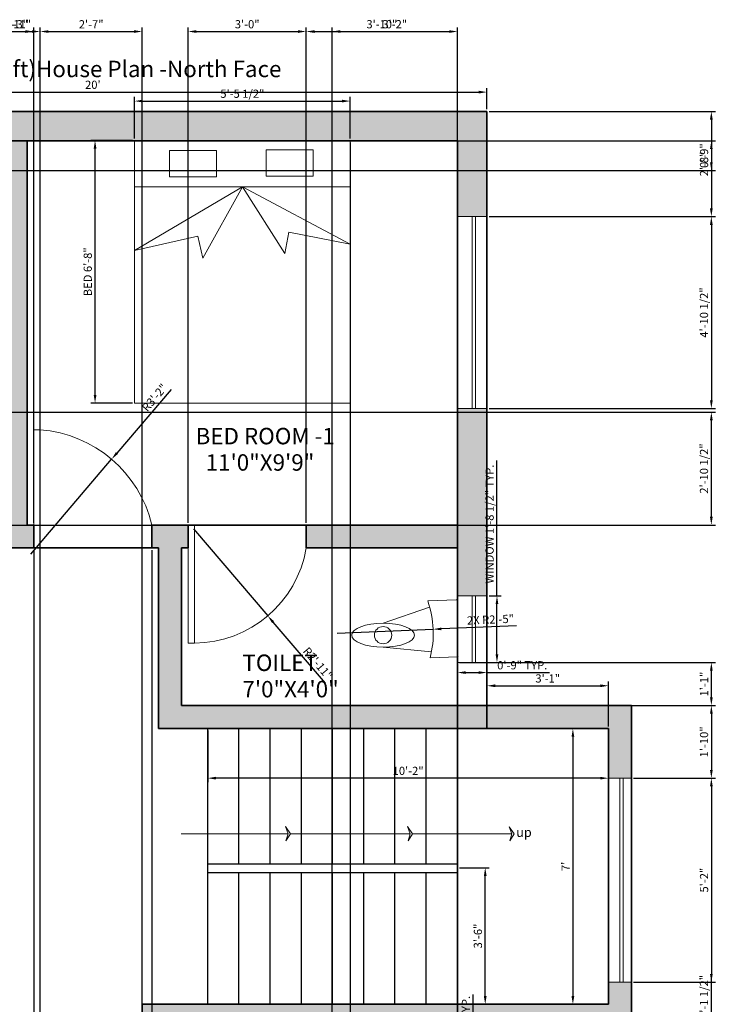
# Model space of a CAD drawing. Units: millimetres. Extents: x 2466 to 2817, y 2000 to 2512.
# Tile 4 of 4: x 2605 to 2817, y 2210 to 2510. Entities that reach past the tile are written whole.
import ezdxf

# ---------------------------------------------------------------- set-up
doc = ezdxf.new("R2010")
doc.units = ezdxf.units.MM
for name, color, linetype, lineweight in [('A-ANNO-DIMS', 2, 'Continuous', 13), ('A-ANNO-SYMB', 1, 'Continuous', 18), ('A-ANNO-TEXT', 7, 'Continuous', 18), ('A-AREA-IDEN', 7, 'Continuous', 18), ('A-DOOR', 3, 'Continuous', 18), ('A-FLOR-FIXT', 9, 'Continuous', 18), ('A-FLOR-STRS', 7, 'Continuous', 25), ('A-FURN', 8, 'Continuous', 18), ('A-GLAZ', 5, 'Continuous', 18), ('A-WALL', 7, 'Continuous', 35), ('A-WALL-PATT', 8, 'Continuous', 13)]:
    doc.layers.add(name, color=color, linetype=linetype, lineweight=lineweight)
doc.styles.get("Standard").update_dxf_attribs({"font": 'arial.ttf'})
doc.dimstyles.new('ISO-25', dxfattribs={"dimtxt": 2.5, "dimasz": 2.5, "dimexe": 1.25, "dimexo": 0.625, "dimtad": 1, "dimdec": 0, "dimlunit": 3, "dimtxsty": 'Standard', "dimcen": 2.5, "dimadec": 0, "dimazin": 0, "dimtfac": 1, "dimtdec": 0, "dimtmove": 0, "dimatfit": 3, "dimfxl": 1, "dimarcsym": 0})

# ---------------------------------------------------------------- blocks, each defined once
blk = doc.blocks.new('MODERN BED')
at = {"color": 0}
for p, q in [((-79.02, 96.24), (0, 96.24)), ((-79.02, 0), (-79.02, 96.24)), ((0, 96.24), (0, 0)), ((0, 79.26), (-79.02, 79.26)), ((-39.51, 79.26), (-79.02, 55.87)), ((-53.99, 53.1), (-39.51, 79.26)), ((-39.51, 79.26), (0, 58.21)), ((-23.98, 54.83), (-39.51, 79.26)), ((-22.46, 62.6), (-23.98, 54.83)), ((0, 58.21), (-22.46, 62.6)), ((-79.02, 55.87), (-55.81, 61.13)), ((-55.81, 61.13), (-53.99, 53.1)), ((0, 0), (-79.02, 0))]:
    blk.add_line(p, q, dxfattribs=at)
for points in [[(-66.19, 92.55), (-48.93, 92.55), (-48.93, 82.91), (-66.19, 82.91)], [(-30.8, 92.85), (-13.54, 92.85), (-13.54, 83.2), (-30.8, 83.2)], [(-30.8, 92.85), (-13.54, 92.85), (-13.54, 83.2), (-30.8, 83.2)]]:
    blk.add_lwpolyline(points, close=True, dxfattribs=at)
blk = doc.blocks.new('*D5')
at = {"layer": 'A-ANNO-DIMS', "color": 0, "lineweight": -2, "transparency": 16777216}
for p, q in [((2738.81, 2251.75), (2747.91, 2251.75)), ((2746.66, 2212.65), (2746.66, 2249.25)), ((2738.81, 2210.15), (2747.91, 2210.15))]:
    blk.add_line(p, q, dxfattribs=at)
at = {"layer": 'A-ANNO-DIMS', "color": 0, "transparency": 16777216}
for points in [[(2746.25, 2249.25), (2747.08, 2249.25), (2746.66, 2251.75)], [(2746.25, 2212.65), (2747.08, 2212.65), (2746.66, 2210.15)]]:
    blk.add_solid(points, dxfattribs=at)
at = {"layer": 'Defpoints', "color": 0, "transparency": 16777216}
for p in [(2738.19, 2251.75), (2746.66, 2251.75), (2738.19, 2210.15)]:
    blk.add_point(p, dxfattribs=at)
at = {"layer": 'A-ANNO-DIMS', "color": 0, "transparency": 16777216, "insert": (2744.76, 2230.95), "char_height": 2.5, "attachment_point": 5, "rotation": 90}
blk.add_mtext('3\'-6"', dxfattribs=at)
blk = doc.blocks.new('*D6')
at = {"layer": 'A-ANNO-DIMS', "color": 0, "lineweight": -2, "transparency": 16777216}
for p, q in [((2783.56, 2294.15), (2772.1, 2294.15)), ((2773.35, 2291.65), (2773.35, 2212.65)), ((2783.56, 2210.15), (2772.1, 2210.15))]:
    blk.add_line(p, q, dxfattribs=at)
at = {"layer": 'A-ANNO-DIMS', "color": 0, "transparency": 16777216}
for points in [[(2772.94, 2291.65), (2773.77, 2291.65), (2773.35, 2294.15)], [(2772.94, 2212.65), (2773.77, 2212.65), (2773.35, 2210.15)]]:
    blk.add_solid(points, dxfattribs=at)
at = {"layer": 'Defpoints', "color": 0, "transparency": 16777216}
for p in [(2784.19, 2294.15), (2773.35, 2210.15), (2784.19, 2210.15)]:
    blk.add_point(p, dxfattribs=at)
at = {"layer": 'A-ANNO-DIMS', "color": 0, "transparency": 16777216, "insert": (2771.48, 2252.15), "char_height": 2.5, "attachment_point": 5, "rotation": 90}
blk.add_mtext("7'", dxfattribs=at)
blk = doc.blocks.new('*D7')
at = {"layer": 'A-ANNO-DIMS', "color": 0, "lineweight": -2, "transparency": 16777216}
for p, q in [((2747.19, 2294.77), (2747.19, 2308.43)), ((2749.69, 2307.18), (2781.69, 2307.18)), ((2784.19, 2294.77), (2784.19, 2308.43))]:
    blk.add_line(p, q, dxfattribs=at)
at = {"layer": 'A-ANNO-DIMS', "color": 0, "transparency": 16777216}
for points in [[(2749.69, 2307.6), (2749.69, 2306.77), (2747.19, 2307.18)], [(2781.69, 2307.6), (2781.69, 2306.77), (2784.19, 2307.18)]]:
    blk.add_solid(points, dxfattribs=at)
at = {"layer": 'Defpoints', "color": 0, "transparency": 16777216}
for p in [(2784.19, 2307.18), (2747.19, 2294.15), (2784.19, 2294.15)]:
    blk.add_point(p, dxfattribs=at)
at = {"layer": 'A-ANNO-DIMS', "color": 0, "transparency": 16777216, "insert": (2765.69, 2309.09), "char_height": 2.5, "attachment_point": 5}
blk.add_mtext('3\'-1"', dxfattribs=at)
blk = doc.blocks.new('*D8')
at = {"layer": 'A-ANNO-DIMS', "color": 0, "lineweight": -2, "transparency": 16777216}
for p, q in [((2662.19, 2293.52), (2662.19, 2277.78)), ((2784.19, 2293.52), (2784.19, 2277.78)), ((2781.69, 2279.03), (2664.69, 2279.03))]:
    blk.add_line(p, q, dxfattribs=at)
at = {"layer": 'A-ANNO-DIMS', "color": 0, "transparency": 16777216}
for points in [[(2664.69, 2279.45), (2664.69, 2278.62), (2662.19, 2279.03)], [(2781.69, 2279.45), (2781.69, 2278.62), (2784.19, 2279.03)]]:
    blk.add_solid(points, dxfattribs=at)
at = {"layer": 'Defpoints', "color": 0, "transparency": 16777216}
for p in [(2662.19, 2294.15), (2784.19, 2294.15), (2662.19, 2279.03)]:
    blk.add_point(p, dxfattribs=at)
at = {"layer": 'A-ANNO-DIMS', "color": 0, "transparency": 16777216, "insert": (2723.19, 2280.93), "char_height": 2.5, "attachment_point": 5}
blk.add_mtext('10\'-2"', dxfattribs=at)
blk = doc.blocks.new('*D9')
at = {"layer": 'A-ANNO-DIMS', "color": 0, "lineweight": -2, "transparency": 16777216}
for p, q in [((2507.19, 2482.77), (2507.19, 2489.26)), ((2509.69, 2488.01), (2744.69, 2488.01)), ((2747.19, 2482.77), (2747.19, 2489.26))]:
    blk.add_line(p, q, dxfattribs=at)
at = {"layer": 'A-ANNO-DIMS', "color": 0, "transparency": 16777216}
for points in [[(2509.69, 2488.43), (2509.69, 2487.6), (2507.19, 2488.01)], [(2744.69, 2488.43), (2744.69, 2487.6), (2747.19, 2488.01)]]:
    blk.add_solid(points, dxfattribs=at)
at = {"layer": 'Defpoints', "color": 0, "transparency": 16777216}
for p in [(2747.19, 2488.01), (2507.19, 2482.15), (2747.19, 2482.15)]:
    blk.add_point(p, dxfattribs=at)
at = {"layer": 'A-ANNO-DIMS', "color": 0, "transparency": 16777216, "insert": (2627.19, 2489.92), "char_height": 2.5, "attachment_point": 5}
blk.add_mtext("20'", dxfattribs=at)
blk = doc.blocks.new('*D10')
at = {"layer": 'A-ANNO-DIMS', "color": 0, "lineweight": -2, "transparency": 16777216}
for p, q in [((2746.56, 2482.15), (2467.98, 2482.15)), ((2469.23, 2479.65), (2469.23, 2028.65)), ((2746.56, 2026.15), (2467.98, 2026.15))]:
    blk.add_line(p, q, dxfattribs=at)
at = {"layer": 'A-ANNO-DIMS', "color": 0, "transparency": 16777216}
for points in [[(2468.82, 2479.65), (2469.65, 2479.65), (2469.23, 2482.15)], [(2468.82, 2028.65), (2469.65, 2028.65), (2469.23, 2026.15)]]:
    blk.add_solid(points, dxfattribs=at)
at = {"layer": 'Defpoints', "color": 0, "transparency": 16777216}
for p in [(2747.19, 2482.15), (2469.23, 2026.15), (2747.19, 2026.15)]:
    blk.add_point(p, dxfattribs=at)
at = {"layer": 'A-ANNO-DIMS', "color": 0, "transparency": 16777216, "insert": (2467.33, 2254.15), "char_height": 2.5, "attachment_point": 5, "rotation": 90}
blk.add_mtext("38'", dxfattribs=at)
blk = doc.blocks.new('WC-PLAN')
for p, q in [((23.74, 15.5), (9.57, 10.55)), ((23.15, 17.36), (31.83, 17.72)), ((24.29, 1.87), (9.58, 3.3)), ((32.19, 0.34), (23.86, 0))]:
    blk.add_line(p, q)
blk.add_circle((9.58, 6.93), 2.64)
blk.add_arc((-4.38, 7.53), 29.23, 345.0736, 19.6488)
blk.add_ellipse((9.58, 6.93), major_axis=(9.58, 0.01), ratio=0.378572)
blk = doc.blocks.new('WIN-BATH')
for p, q in [((4.5, 20.33), (4.5, 0)), ((5.5, 20.33), (5.5, 0))]:
    blk.add_line(p, q)
blk.add_lwpolyline([(9, 20.33), (0, 20.33), (0, 0), (9, 0)], close=True)
blk = doc.blocks.new('STAIR-DIRECTION-HEAD')
blk.add_lwpolyline([(0, 4.35), (0.84, 2.19), (0.16, 0), (1.53, 2.19)], close=True)
blk = doc.blocks.new('*D18')
at = {"layer": 'A-ANNO-DIMS', "color": 0, "lineweight": -2, "transparency": 16777216}
for p, q in [((2750.24, 2334.57), (2750.24, 2375.78)), ((2747.81, 2334.57), (2751.49, 2334.57)), ((2750.24, 2316.74), (2750.24, 2332.07)), ((2747.81, 2314.24), (2751.49, 2314.24))]:
    blk.add_line(p, q, dxfattribs=at)
at = {"layer": 'A-ANNO-DIMS', "color": 0, "transparency": 16777216}
for points in [[(2749.82, 2332.07), (2750.65, 2332.07), (2750.24, 2334.57)], [(2749.82, 2316.74), (2750.65, 2316.74), (2750.24, 2314.24)]]:
    blk.add_solid(points, dxfattribs=at)
at = {"layer": 'Defpoints', "color": 0, "transparency": 16777216}
for p in [(2747.19, 2334.57), (2750.24, 2334.57), (2747.19, 2314.24)]:
    blk.add_point(p, dxfattribs=at)
at = {"layer": 'A-ANNO-DIMS', "color": 0, "transparency": 16777216, "insert": (2748.32, 2356.43), "char_height": 2.5, "attachment_point": 5, "rotation": 90}
blk.add_mtext('WINDOW 1\'-8 1/2" TYP.', dxfattribs=at)
blk = doc.blocks.new('*D19')
at = {"layer": 'A-ANNO-DIMS', "color": 0, "lineweight": -2, "transparency": 16777216}
for p, q in [((2738.19, 2313.62), (2738.19, 2309.95)), ((2747.19, 2313.62), (2747.19, 2309.95)), ((2740.69, 2311.2), (2744.69, 2311.2)), ((2747.19, 2311.2), (2766.18, 2311.2))]:
    blk.add_line(p, q, dxfattribs=at)
at = {"layer": 'A-ANNO-DIMS', "color": 0, "transparency": 16777216}
for points in [[(2740.69, 2311.61), (2740.69, 2310.78), (2738.19, 2311.2)], [(2744.69, 2311.61), (2744.69, 2310.78), (2747.19, 2311.2)]]:
    blk.add_solid(points, dxfattribs=at)
at = {"layer": 'Defpoints', "color": 0, "transparency": 16777216}
for p in [(2738.19, 2314.24), (2747.19, 2314.24), (2747.19, 2311.2)]:
    blk.add_point(p, dxfattribs=at)
at = {"layer": 'A-ANNO-DIMS', "color": 0, "transparency": 16777216, "insert": (2757.93, 2313.1), "char_height": 2.5, "attachment_point": 5}
blk.add_mtext('0\'-9" TYP.', dxfattribs=at)
blk = doc.blocks.new('*D21')
at = {"layer": 'A-ANNO-DIMS', "color": 0, "lineweight": -2, "transparency": 16777216}
for p, q in [((2743.02, 2188.59), (2743.02, 2213.17)), ((2738.81, 2188.59), (2744.27, 2188.59)), ((2743.02, 2173.37), (2743.02, 2186.09)), ((2738.81, 2170.87), (2744.27, 2170.87))]:
    blk.add_line(p, q, dxfattribs=at)
at = {"layer": 'A-ANNO-DIMS', "color": 0, "transparency": 16777216}
for points in [[(2742.6, 2186.09), (2743.43, 2186.09), (2743.02, 2188.59)], [(2742.6, 2173.37), (2743.43, 2173.37), (2743.02, 2170.87)]]:
    blk.add_solid(points, dxfattribs=at)
at = {"layer": 'Defpoints', "color": 0, "transparency": 16777216}
for p in [(2738.19, 2188.59), (2743.02, 2188.59), (2738.19, 2170.87)]:
    blk.add_point(p, dxfattribs=at)
at = {"layer": 'A-ANNO-DIMS', "color": 0, "transparency": 16777216, "insert": (2741.1, 2202.13), "char_height": 2.5, "attachment_point": 5, "rotation": 90}
blk.add_mtext('1\'-5 1/2" TYP.', dxfattribs=at)
blk = doc.blocks.new('*D24')
at = {"layer": 'A-ANNO-DIMS', "color": 0, "lineweight": -2, "transparency": 16777216}
for p, q in [((2639.25, 2473.28), (2626.62, 2473.28)), ((2627.87, 2395.78), (2627.87, 2470.78)), ((2639.25, 2393.28), (2626.62, 2393.28))]:
    blk.add_line(p, q, dxfattribs=at)
at = {"layer": 'A-ANNO-DIMS', "color": 0, "transparency": 16777216}
for points in [[(2627.45, 2470.78), (2628.29, 2470.78), (2627.87, 2473.28)], [(2627.45, 2395.78), (2628.29, 2395.78), (2627.87, 2393.28)]]:
    blk.add_solid(points, dxfattribs=at)
at = {"layer": 'Defpoints', "color": 0, "transparency": 16777216}
for p in [(2627.87, 2473.28), (2639.87, 2473.28), (2639.87, 2393.28)]:
    blk.add_point(p, dxfattribs=at)
at = {"layer": 'A-ANNO-DIMS', "color": 0, "transparency": 16777216, "insert": (2625.97, 2433.28), "char_height": 2.5, "attachment_point": 5, "rotation": 90}
blk.add_mtext('BED 6\'-8"', dxfattribs=at)
blk = doc.blocks.new('*D25')
at = {"layer": 'A-ANNO-DIMS', "color": 0, "lineweight": -2, "transparency": 16777216}
for p, q in [((2639.87, 2473.91), (2639.87, 2486.53)), ((2705.56, 2473.91), (2705.56, 2486.53)), ((2642.37, 2485.28), (2703.06, 2485.28))]:
    blk.add_line(p, q, dxfattribs=at)
at = {"layer": 'A-ANNO-DIMS', "color": 0, "transparency": 16777216}
for points in [[(2642.37, 2485.7), (2642.37, 2484.87), (2639.87, 2485.28)], [(2703.06, 2485.7), (2703.06, 2484.87), (2705.56, 2485.28)]]:
    blk.add_solid(points, dxfattribs=at)
at = {"layer": 'Defpoints', "color": 0, "transparency": 16777216}
for p in [(2705.56, 2485.28), (2639.87, 2473.28), (2705.56, 2473.28)]:
    blk.add_point(p, dxfattribs=at)
at = {"layer": 'A-ANNO-DIMS', "color": 0, "transparency": 16777216, "insert": (2672.72, 2487.2), "char_height": 2.5, "attachment_point": 5}
blk.add_mtext('5\'-5 1/2"', dxfattribs=at)
blk = doc.blocks.new('*D36')
at = {"layer": 'A-ANNO-DIMS', "color": 0, "lineweight": -2, "transparency": 16777216}
for p, q in [((2747.81, 2482.15), (2816.76, 2482.15)), ((2815.51, 2479.65), (2815.51, 2452.58)), ((2747.81, 2450.08), (2816.76, 2450.08))]:
    blk.add_line(p, q, dxfattribs=at)
at = {"layer": 'A-ANNO-DIMS', "color": 0, "transparency": 16777216}
for points in [[(2815.09, 2479.65), (2815.92, 2479.65), (2815.51, 2482.15)], [(2815.09, 2452.58), (2815.92, 2452.58), (2815.51, 2450.08)]]:
    blk.add_solid(points, dxfattribs=at)
at = {"layer": 'Defpoints', "color": 0, "transparency": 16777216}
for p in [(2747.19, 2482.15), (2747.19, 2450.08), (2815.51, 2450.08)]:
    blk.add_point(p, dxfattribs=at)
at = {"layer": 'A-ANNO-DIMS', "color": 0, "transparency": 16777216, "insert": (2813.61, 2466.12), "char_height": 2.5, "attachment_point": 5, "rotation": 90}
blk.add_mtext('2\'-8"', dxfattribs=at)
blk = doc.blocks.new('*D37')
at = {"layer": 'A-ANNO-DIMS', "color": 0, "lineweight": -2, "transparency": 16777216}
for p, q in [((2747.81, 2450.08), (2816.76, 2450.08)), ((2815.51, 2447.58), (2815.51, 2394.15)), ((2747.81, 2391.65), (2816.76, 2391.65))]:
    blk.add_line(p, q, dxfattribs=at)
at = {"layer": 'A-ANNO-DIMS', "color": 0, "transparency": 16777216}
for points in [[(2815.09, 2447.58), (2815.92, 2447.58), (2815.51, 2450.08)], [(2815.09, 2394.15), (2815.92, 2394.15), (2815.51, 2391.65)]]:
    blk.add_solid(points, dxfattribs=at)
at = {"layer": 'Defpoints', "color": 0, "transparency": 16777216}
for p in [(2747.19, 2450.08), (2747.19, 2391.65), (2815.51, 2391.65)]:
    blk.add_point(p, dxfattribs=at)
at = {"layer": 'A-ANNO-DIMS', "color": 0, "transparency": 16777216, "insert": (2813.59, 2420.87), "char_height": 2.5, "attachment_point": 5, "rotation": 90}
blk.add_mtext('4\'-10 1/2"', dxfattribs=at)
blk = doc.blocks.new('*D38')
at = {"layer": 'A-ANNO-DIMS', "color": 0, "lineweight": -2, "transparency": 16777216}
for p, q in [((2791.81, 2301.15), (2816.76, 2301.15)), ((2815.51, 2298.65), (2815.51, 2281.53)), ((2791.81, 2279.03), (2816.76, 2279.03))]:
    blk.add_line(p, q, dxfattribs=at)
at = {"layer": 'A-ANNO-DIMS', "color": 0, "transparency": 16777216}
for points in [[(2815.09, 2298.65), (2815.92, 2298.65), (2815.51, 2301.15)], [(2815.09, 2281.53), (2815.92, 2281.53), (2815.51, 2279.03)]]:
    blk.add_solid(points, dxfattribs=at)
at = {"layer": 'Defpoints', "color": 0, "transparency": 16777216}
for p in [(2791.19, 2301.15), (2791.19, 2279.03), (2815.51, 2279.03)]:
    blk.add_point(p, dxfattribs=at)
at = {"layer": 'A-ANNO-DIMS', "color": 0, "transparency": 16777216, "insert": (2813.61, 2290.09), "char_height": 2.5, "attachment_point": 5, "rotation": 90}
blk.add_mtext('1\'-10"', dxfattribs=at)
blk = doc.blocks.new('*D39')
at = {"layer": 'A-ANNO-DIMS', "color": 0, "lineweight": -2, "transparency": 16777216}
for p, q in [((2791.81, 2279.03), (2816.76, 2279.03)), ((2815.51, 2276.53), (2815.51, 2219.4)), ((2791.81, 2216.9), (2816.76, 2216.9))]:
    blk.add_line(p, q, dxfattribs=at)
at = {"layer": 'A-ANNO-DIMS', "color": 0, "transparency": 16777216}
for points in [[(2815.09, 2276.53), (2815.92, 2276.53), (2815.51, 2279.03)], [(2815.09, 2219.4), (2815.92, 2219.4), (2815.51, 2216.9)]]:
    blk.add_solid(points, dxfattribs=at)
at = {"layer": 'Defpoints', "color": 0, "transparency": 16777216}
for p in [(2791.19, 2279.03), (2791.19, 2216.9), (2815.51, 2216.9)]:
    blk.add_point(p, dxfattribs=at)
at = {"layer": 'A-ANNO-DIMS', "color": 0, "transparency": 16777216, "insert": (2813.61, 2247.97), "char_height": 2.5, "attachment_point": 5, "rotation": 90}
blk.add_mtext('5\'-2"', dxfattribs=at)
blk = doc.blocks.new('*D43')
at = {"layer": 'A-ANNO-DIMS', "color": 0, "lineweight": -2, "transparency": 16777216}
for p, q in [((2700.05, 2035.77), (2700.05, 2507.72)), ((2738.19, 2035.77), (2738.19, 2507.72)), ((2702.55, 2506.47), (2735.69, 2506.47))]:
    blk.add_line(p, q, dxfattribs=at)
at = {"layer": 'A-ANNO-DIMS', "color": 0, "transparency": 16777216}
for points in [[(2702.55, 2506.88), (2702.55, 2506.05), (2700.05, 2506.47)], [(2735.69, 2506.88), (2735.69, 2506.05), (2738.19, 2506.47)]]:
    blk.add_solid(points, dxfattribs=at)
at = {"layer": 'Defpoints', "color": 0, "transparency": 16777216}
for p in [(2738.19, 2506.47), (2700.05, 2035.15), (2738.19, 2035.15)]:
    blk.add_point(p, dxfattribs=at)
at = {"layer": 'A-ANNO-DIMS', "color": 0, "transparency": 16777216, "insert": (2719.12, 2508.37), "char_height": 2.5, "attachment_point": 5}
blk.add_mtext('3\'-2"', dxfattribs=at)
blk = doc.blocks.new('*D49')
at = {"layer": 'A-ANNO-DIMS', "color": 0, "lineweight": -2, "transparency": 16777216}
for p, q in [((2598.19, 2356.77), (2598.19, 2507.72)), ((2609.19, 2356.77), (2609.19, 2507.72)), ((2600.69, 2506.47), (2606.69, 2506.47))]:
    blk.add_line(p, q, dxfattribs=at)
at = {"layer": 'A-ANNO-DIMS', "color": 0, "transparency": 16777216}
for points in [[(2600.69, 2506.88), (2600.69, 2506.05), (2598.19, 2506.47)], [(2606.69, 2506.88), (2606.69, 2506.05), (2609.19, 2506.47)]]:
    blk.add_solid(points, dxfattribs=at)
at = {"layer": 'Defpoints', "color": 0, "transparency": 16777216}
for p in [(2609.19, 2506.47), (2598.19, 2356.15), (2609.19, 2356.15)]:
    blk.add_point(p, dxfattribs=at)
at = {"layer": 'A-ANNO-DIMS', "color": 0, "transparency": 16777216, "insert": (2603.69, 2508.37), "char_height": 2.5, "attachment_point": 5}
blk.add_mtext('0\'-11"', dxfattribs=at)
blk = doc.blocks.new('*D50')
at = {"layer": 'A-ANNO-DIMS', "color": 0, "lineweight": -2, "transparency": 16777216}
for p, q in [((2609.19, 2348.52), (2609.19, 2000.58)), ((2645.19, 2348.52), (2645.19, 2000.58)), ((2611.69, 2001.83), (2642.69, 2001.83))]:
    blk.add_line(p, q, dxfattribs=at)
at = {"layer": 'A-ANNO-DIMS', "color": 0, "transparency": 16777216}
for points in [[(2611.69, 2002.24), (2611.69, 2001.41), (2609.19, 2001.83)], [(2642.69, 2002.24), (2642.69, 2001.41), (2645.19, 2001.83)]]:
    blk.add_solid(points, dxfattribs=at)
at = {"layer": 'Defpoints', "color": 0, "transparency": 16777216}
for p in [(2609.19, 2349.15), (2645.19, 2349.15), (2645.19, 2001.83)]:
    blk.add_point(p, dxfattribs=at)
at = {"layer": 'A-ANNO-DIMS', "color": 0, "transparency": 16777216, "insert": (2627.19, 2003.73), "char_height": 2.5, "attachment_point": 5}
blk.add_mtext('3\'-0"', dxfattribs=at)
blk = doc.blocks.new('*D53')
at = {"layer": 'A-ANNO-DIMS', "color": 0, "lineweight": -2, "transparency": 16777216}
for p, q in [((2596.19, 2155.77), (2596.19, 2507.72)), ((2611.19, 2155.77), (2611.19, 2507.72)), ((2598.69, 2506.47), (2608.69, 2506.47))]:
    blk.add_line(p, q, dxfattribs=at)
at = {"layer": 'A-ANNO-DIMS', "color": 0, "transparency": 16777216}
for points in [[(2598.69, 2506.88), (2598.69, 2506.05), (2596.19, 2506.47)], [(2608.69, 2506.88), (2608.69, 2506.05), (2611.19, 2506.47)]]:
    blk.add_solid(points, dxfattribs=at)
at = {"layer": 'Defpoints', "color": 0, "transparency": 16777216}
for p in [(2611.19, 2506.47), (2596.19, 2155.15), (2611.19, 2155.15)]:
    blk.add_point(p, dxfattribs=at)
at = {"layer": 'A-ANNO-DIMS', "color": 0, "transparency": 16777216, "insert": (2603.69, 2508.37), "char_height": 2.5, "attachment_point": 5}
blk.add_mtext('1\'-3"', dxfattribs=at)
blk = doc.blocks.new('*D54')
at = {"layer": 'A-ANNO-DIMS', "color": 0, "lineweight": -2, "transparency": 16777216}
for p, q in [((2611.19, 2155.77), (2611.19, 2507.72)), ((2642.19, 2155.77), (2642.19, 2507.72)), ((2613.69, 2506.47), (2639.69, 2506.47))]:
    blk.add_line(p, q, dxfattribs=at)
at = {"layer": 'A-ANNO-DIMS', "color": 0, "transparency": 16777216}
for points in [[(2613.69, 2506.88), (2613.69, 2506.05), (2611.19, 2506.47)], [(2639.69, 2506.88), (2639.69, 2506.05), (2642.19, 2506.47)]]:
    blk.add_solid(points, dxfattribs=at)
at = {"layer": 'Defpoints', "color": 0, "transparency": 16777216}
for p in [(2642.19, 2506.47), (2611.19, 2155.15), (2642.19, 2155.15)]:
    blk.add_point(p, dxfattribs=at)
at = {"layer": 'A-ANNO-DIMS', "color": 0, "transparency": 16777216, "insert": (2626.69, 2508.35), "char_height": 2.5, "attachment_point": 5}
blk.add_mtext('2\'-7"', dxfattribs=at)
blk = doc.blocks.new('*D57')
at = {"layer": 'A-ANNO-DIMS', "color": 0, "lineweight": -2, "transparency": 16777216}
for p, q in [((2815.51, 2203.15), (2815.51, 2219.13)), ((2747.81, 2203.15), (2816.76, 2203.15)), ((2815.51, 2192.2), (2815.51, 2200.65)), ((2747.81, 2189.7), (2816.76, 2189.7))]:
    blk.add_line(p, q, dxfattribs=at)
at = {"layer": 'A-ANNO-DIMS', "color": 0, "transparency": 16777216}
for points in [[(2815.09, 2200.65), (2815.92, 2200.65), (2815.51, 2203.15)], [(2815.09, 2192.2), (2815.92, 2192.2), (2815.51, 2189.7)]]:
    blk.add_solid(points, dxfattribs=at)
at = {"layer": 'Defpoints', "color": 0, "transparency": 16777216}
for p in [(2747.19, 2203.15), (2815.51, 2203.15), (2747.19, 2189.7)]:
    blk.add_point(p, dxfattribs=at)
at = {"layer": 'A-ANNO-DIMS', "color": 0, "transparency": 16777216, "insert": (2813.59, 2212.39), "char_height": 2.5, "attachment_point": 5, "rotation": 90}
blk.add_mtext('1\'-1 1/2"', dxfattribs=at)
blk = doc.blocks.new('*D58')
at = {"layer": 'A-ANNO-DIMS', "color": 0, "lineweight": -2, "transparency": 16777216}
for p, q in [((2738.81, 2314.24), (2816.76, 2314.24)), ((2815.51, 2303.65), (2815.51, 2311.74)), ((2738.81, 2301.15), (2816.76, 2301.15))]:
    blk.add_line(p, q, dxfattribs=at)
at = {"layer": 'A-ANNO-DIMS', "color": 0, "transparency": 16777216}
for points in [[(2815.09, 2311.74), (2815.92, 2311.74), (2815.51, 2314.24)], [(2815.09, 2303.65), (2815.92, 2303.65), (2815.51, 2301.15)]]:
    blk.add_solid(points, dxfattribs=at)
at = {"layer": 'Defpoints', "color": 0, "transparency": 16777216}
for p in [(2738.19, 2314.24), (2815.51, 2314.24), (2738.19, 2301.15)]:
    blk.add_point(p, dxfattribs=at)
at = {"layer": 'A-ANNO-DIMS', "color": 0, "transparency": 16777216, "insert": (2813.63, 2307.7), "char_height": 2.5, "attachment_point": 5, "rotation": 90}
blk.add_mtext('1\'-1"', dxfattribs=at)
blk = doc.blocks.new('*D60')
at = {"layer": 'A-ANNO-DIMS', "color": 0, "lineweight": -2, "transparency": 16777216}
for p, q in [((2656.19, 2356.77), (2656.19, 2507.72)), ((2692.19, 2356.77), (2692.19, 2507.72)), ((2658.69, 2506.47), (2689.69, 2506.47))]:
    blk.add_line(p, q, dxfattribs=at)
at = {"layer": 'A-ANNO-DIMS', "color": 0, "transparency": 16777216}
for points in [[(2658.69, 2506.88), (2658.69, 2506.05), (2656.19, 2506.47)], [(2689.69, 2506.88), (2689.69, 2506.05), (2692.19, 2506.47)]]:
    blk.add_solid(points, dxfattribs=at)
at = {"layer": 'Defpoints', "color": 0, "transparency": 16777216}
for p in [(2692.19, 2506.47), (2656.19, 2356.15), (2692.19, 2356.15)]:
    blk.add_point(p, dxfattribs=at)
at = {"layer": 'A-ANNO-DIMS', "color": 0, "transparency": 16777216, "insert": (2674.19, 2508.37), "char_height": 2.5, "attachment_point": 5}
blk.add_mtext('3\'-0"', dxfattribs=at)
blk = doc.blocks.new('*D61')
at = {"layer": 'A-ANNO-DIMS', "color": 0, "lineweight": -2, "transparency": 16777216}
for p, q in [((2692.19, 2356.77), (2692.19, 2507.72)), ((2738.19, 2356.77), (2738.19, 2507.72)), ((2694.69, 2506.47), (2735.69, 2506.47))]:
    blk.add_line(p, q, dxfattribs=at)
at = {"layer": 'A-ANNO-DIMS', "color": 0, "transparency": 16777216}
for points in [[(2694.69, 2506.88), (2694.69, 2506.05), (2692.19, 2506.47)], [(2735.69, 2506.88), (2735.69, 2506.05), (2738.19, 2506.47)]]:
    blk.add_solid(points, dxfattribs=at)
at = {"layer": 'Defpoints', "color": 0, "transparency": 16777216}
for p in [(2738.19, 2506.47), (2692.19, 2356.15), (2738.19, 2356.15)]:
    blk.add_point(p, dxfattribs=at)
at = {"layer": 'A-ANNO-DIMS', "color": 0, "transparency": 16777216, "insert": (2715.19, 2508.37), "char_height": 2.5, "attachment_point": 5}
blk.add_mtext('3\'-10"', dxfattribs=at)
blk = doc.blocks.new('*D67')
at = {"layer": 'A-ANNO-DIMS', "color": 0, "lineweight": -2, "transparency": 16777216}
for p, q in [((2705.56, 2472.66), (2705.56, 2000.58)), ((2738.19, 2472.52), (2738.19, 2000.58)), ((2708.06, 2001.83), (2735.69, 2001.83))]:
    blk.add_line(p, q, dxfattribs=at)
at = {"layer": 'A-ANNO-DIMS', "color": 0, "transparency": 16777216}
for points in [[(2708.06, 2002.24), (2708.06, 2001.41), (2705.56, 2001.83)], [(2735.69, 2002.24), (2735.69, 2001.41), (2738.19, 2001.83)]]:
    blk.add_solid(points, dxfattribs=at)
at = {"layer": 'Defpoints', "color": 0, "transparency": 16777216}
for p in [(2705.56, 2473.28), (2738.19, 2473.15), (2738.19, 2001.83)]:
    blk.add_point(p, dxfattribs=at)
at = {"layer": 'A-ANNO-DIMS', "color": 0, "transparency": 16777216, "insert": (2721.87, 2003.75), "char_height": 2.5, "attachment_point": 5}
blk.add_mtext('2\'-8 1/2"', dxfattribs=at)
blk = doc.blocks.new('*D70')
at = {"layer": 'A-ANNO-DIMS', "color": 0, "lineweight": -2, "transparency": 16777216}
for p, q in [((2524.58, 2390.56), (2816.76, 2390.56)), ((2815.51, 2358.65), (2815.51, 2388.06)), ((2516.81, 2356.15), (2816.76, 2356.15))]:
    blk.add_line(p, q, dxfattribs=at)
at = {"layer": 'A-ANNO-DIMS', "color": 0, "transparency": 16777216}
for points in [[(2815.09, 2388.06), (2815.92, 2388.06), (2815.51, 2390.56)], [(2815.09, 2358.65), (2815.92, 2358.65), (2815.51, 2356.15)]]:
    blk.add_solid(points, dxfattribs=at)
at = {"layer": 'Defpoints', "color": 0, "transparency": 16777216}
for p in [(2523.95, 2390.56), (2815.51, 2390.56), (2516.19, 2356.15)]:
    blk.add_point(p, dxfattribs=at)
at = {"layer": 'A-ANNO-DIMS', "color": 0, "transparency": 16777216, "insert": (2813.59, 2373.35), "char_height": 2.5, "attachment_point": 5, "rotation": 90}
blk.add_mtext('2\'-10 1/2"', dxfattribs=at)
blk = doc.blocks.new('*D72')
at = {"layer": 'A-ANNO-DIMS', "color": 0, "lineweight": -2, "transparency": 16777216}
for p, q in [((2589.71, 2473.15), (2816.76, 2473.15)), ((2815.51, 2470.65), (2815.51, 2466.64)), ((2587.82, 2464.14), (2816.76, 2464.14))]:
    blk.add_line(p, q, dxfattribs=at)
at = {"layer": 'A-ANNO-DIMS', "color": 0, "transparency": 16777216}
for points in [[(2815.09, 2470.65), (2815.92, 2470.65), (2815.51, 2473.15)], [(2815.09, 2466.64), (2815.92, 2466.64), (2815.51, 2464.14)]]:
    blk.add_solid(points, dxfattribs=at)
at = {"layer": 'Defpoints', "color": 0, "transparency": 16777216}
for p in [(2589.08, 2473.15), (2587.19, 2464.14), (2815.51, 2464.14)]:
    blk.add_point(p, dxfattribs=at)
at = {"layer": 'A-ANNO-DIMS', "color": 0, "transparency": 16777216, "insert": (2813.61, 2468.65), "char_height": 2.5, "attachment_point": 5, "rotation": 90}
blk.add_mtext('0\'-9"', dxfattribs=at)
blk = doc.blocks.new('*D74')
at = {"layer": 'A-ANNO-DIMS', "color": 0, "lineweight": -2, "transparency": 16777216}
for p, q in [((2651.03, 2397.43), (2634.53, 2378.08)), ((2608.27, 2347.29), (2632.91, 2376.18))]:
    blk.add_line(p, q, dxfattribs=at)
at = {"layer": 'A-ANNO-DIMS', "color": 0, "transparency": 16777216}
blk.add_solid([(2634.21, 2378.35), (2634.84, 2377.81), (2632.91, 2376.18)], dxfattribs=at)
at = {"layer": 'Defpoints', "color": 0, "transparency": 16777216}
for p in [(2632.91, 2376.18), (2608.27, 2347.29)]:
    blk.add_point(p, dxfattribs=at)
at = {"layer": 'A-ANNO-DIMS', "color": 0, "transparency": 16777216, "insert": (2646.24, 2394.75), "char_height": 2.5, "attachment_point": 5, "rotation": 49.5381}
blk.add_mtext('R3\'-2"', dxfattribs=at)
blk = doc.blocks.new('*D76')
at = {"layer": 'A-ANNO-DIMS', "color": 0, "lineweight": -2, "transparency": 16777216}
for p, q in [((2657.85, 2354.97), (2680.45, 2328.48)), ((2697.98, 2307.93), (2682.07, 2326.57))]:
    blk.add_line(p, q, dxfattribs=at)
at = {"layer": 'A-ANNO-DIMS', "color": 0, "transparency": 16777216}
blk.add_solid([(2682.39, 2326.84), (2681.76, 2326.3), (2680.45, 2328.48)], dxfattribs=at)
at = {"layer": 'Defpoints', "color": 0, "transparency": 16777216}
for p in [(2657.85, 2354.97), (2680.45, 2328.48)]:
    blk.add_point(p, dxfattribs=at)
at = {"layer": 'A-ANNO-DIMS', "color": 0, "transparency": 16777216, "insert": (2695.44, 2313.8), "char_height": 2.5, "attachment_point": 5, "rotation": 310.4623}
blk.add_mtext('R2\'-11"', dxfattribs=at)
blk = doc.blocks.new('*D80')
at = {"layer": 'A-ANNO-DIMS', "color": 0, "lineweight": -2, "transparency": 16777216}
for p, q in [((2756.19, 2325.44), (2733.32, 2324.5)), ((2701.61, 2323.19), (2730.82, 2324.4))]:
    blk.add_line(p, q, dxfattribs=at)
at = {"layer": 'A-ANNO-DIMS', "color": 0, "transparency": 16777216}
blk.add_solid([(2733.3, 2324.91), (2733.34, 2324.08), (2730.82, 2324.4)], dxfattribs=at)
at = {"layer": 'Defpoints', "color": 0, "transparency": 16777216}
for p in [(2701.61, 2323.19), (2730.82, 2324.4)]:
    blk.add_point(p, dxfattribs=at)
at = {"layer": 'A-ANNO-DIMS', "color": 0, "transparency": 16777216, "insert": (2748.27, 2327.02), "char_height": 2.5, "attachment_point": 5, "rotation": 2.3618}
blk.add_mtext('2X R2\'-5"', dxfattribs=at)

msp = doc.modelspace()

# ---------------------------------------------------------------- hatches: boundary and pattern name
at = {"layer": 'A-WALL-PATT'}
h = msp.add_hatch(color=256, dxfattribs=at)
h.dxf.hatch_style = 1
h.paths.add_polyline_path([(2747.19, 2482.15), (2589.08, 2482.15), (2589.08, 2473.15), (2639.87, 2473.15), (2639.87, 2473.28), (2705.56, 2473.28), (2738.19, 2473.15), (2738.19, 2450.08), (2747.19, 2450.08)])
h.paths.add_polyline_path([(2564.77, 2482.15), (2507.19, 2482.15), (2507.19, 2440.79), (2516.19, 2440.79), (2516.19, 2473.15), (2564.77, 2473.15)])
h.paths.add_polyline_path([(2516.19, 2383.84), (2507.19, 2383.84), (2507.19, 2339.92), (2516.19, 2339.92)])
h.paths.add_polyline_path([(2607.19, 2473.15), (2600.19, 2473.15), (2600.19, 2356.15), (2607.19, 2356.15)])
h.paths.add_polyline_path([(2747.19, 2391.65), (2738.19, 2391.65), (2738.19, 2334.57), (2747.19, 2334.57)])
h = msp.add_hatch(color=256, dxfattribs=at)
h.dxf.hatch_style = 1
h.paths.add_polyline_path([(2562.19, 2356.15), (2516.19, 2356.15), (2516.19, 2349.15), (2562.19, 2349.15)])
h.paths.add_polyline_path([(2738.19, 2356.15), (2692.19, 2356.15), (2692.19, 2349.15), (2738.19, 2349.15)], flags=17)
h.paths.add_polyline_path([(2656.19, 2356.15), (2645.19, 2356.15), (2645.19, 2349.15), (2647.19, 2349.15), (2647.19, 2294.15), (2738.19, 2294.15), (2747.19, 2294.15), (2747.19, 2301.15), (2738.19, 2301.15), (2654.19, 2301.15), (2654.19, 2349.15), (2656.19, 2349.15)])
h = msp.add_hatch(color=256, dxfattribs=at)
h.dxf.hatch_style = 1
h.paths.add_polyline_path([(2609.19, 2356.15), (2607.19, 2356.15), (2598.19, 2356.15), (2598.19, 2349.15), (2609.19, 2349.15)])
h = msp.add_hatch(color=256, dxfattribs=at)
h.dxf.hatch_style = 1
h.paths.add_polyline_path([(2791.19, 2301.15), (2747.19, 2301.15), (2747.19, 2294.15), (2784.19, 2294.15), (2784.19, 2279.03), (2791.19, 2279.03)])
h.paths.add_polyline_path([(2791.19, 2216.9), (2784.19, 2216.9), (2784.19, 2210.15), (2662.19, 2210.15), (2647.19, 2210.15), (2645.19, 2210.15), (2642.19, 2210.15), (2642.19, 2203.15), (2646.68, 2203.15), (2646.68, 2193.15), (2653.68, 2193.15), (2653.68, 2203.15), (2654.69, 2203.15), (2662.19, 2203.15), (2791.19, 2203.15)])

# ---------------------------------------------------------------- linework, layer by layer
at = {"layer": 'A-ANNO-SYMB'}
for p, q in [((2654.13, 2262.09), (2686.65, 2262.09)), ((2687.34, 2262.09), (2723.83, 2262.09)), ((2724.51, 2262.09), (2754.81, 2262.09))]:
    msp.add_line(p, q, dxfattribs=at)
at = {"layer": 'A-DOOR'}
for p, q in [((2609.19, 2356.15), (2609.19, 2385.15)), ((2609.19, 2385.15), (2611.19, 2385.15)), ((2611.19, 2385.15), (2611.19, 2349.15)), ((2658.19, 2320.15), (2658.19, 2356.15)), ((2656.19, 2349.15), (2656.19, 2320.15)), ((2656.19, 2320.15), (2658.19, 2320.15))]:
    msp.add_line(p, q, dxfattribs=at)
for centre, radius, start, end in [((2608.27, 2347.29), 37.97, 13.4871, 85.5884), ((2657.85, 2354.97), 34.82, 270.5495, 350.375)]:
    msp.add_arc(centre, radius, start, end, dxfattribs=at)
at = {"layer": 'A-FLOR-FIXT'}
for p, q in [((2737.83, 2333.38), (2738.19, 2333.39)), ((2738.54, 2316.02), (2738.54, 2316.02))]:
    msp.add_line(p, q, dxfattribs=at)
at = {"layer": 'A-FLOR-STRS'}
for p, q in [((2662.19, 2210.15), (2662.19, 2294.15)), ((2671.69, 2252.86), (2671.69, 2294.15)), ((2681.19, 2252.86), (2681.19, 2294.15)), ((2690.69, 2252.86), (2690.69, 2294.15)), ((2700.19, 2252.86), (2700.19, 2294.15)), ((2709.69, 2252.86), (2709.69, 2294.15)), ((2719.19, 2252.86), (2719.19, 2294.15)), ((2728.69, 2252.86), (2728.69, 2294.15)), ((2738.19, 2294.15), (2738.19, 2210.15)), ((2738.19, 2210.15), (2738.19, 2294.15)), ((2738.19, 2252.86), (2662.19, 2252.86)), ((2738.19, 2250.15), (2662.19, 2250.15)), ((2671.69, 2210.15), (2671.69, 2250.15)), ((2681.19, 2210.15), (2681.19, 2250.15)), ((2690.69, 2210.15), (2690.69, 2250.15)), ((2700.19, 2210.15), (2700.19, 2250.15)), ((2709.69, 2210.15), (2709.69, 2250.15)), ((2719.19, 2210.15), (2719.19, 2250.15)), ((2728.69, 2210.15), (2728.69, 2250.15)), ((2738.19, 2210.15), (2738.19, 2252.15))]:
    msp.add_line(p, q, dxfattribs=at)
at = {"layer": 'A-GLAZ'}
for p, q in [((2738.19, 2450.08), (2747.19, 2450.08)), ((2738.19, 2391.65), (2738.19, 2450.08)), ((2742.69, 2450.08), (2742.69, 2391.65)), ((2743.69, 2450.08), (2743.69, 2391.65)), ((2747.19, 2450.08), (2747.19, 2391.65)), ((2747.19, 2391.65), (2738.19, 2391.65)), ((2784.19, 2279.03), (2791.19, 2279.03)), ((2784.19, 2216.9), (2784.19, 2279.03)), ((2787.69, 2279.03), (2787.69, 2216.9)), ((2788.69, 2279.03), (2788.69, 2216.9)), ((2791.19, 2279.03), (2791.19, 2216.9)), ((2791.19, 2216.9), (2784.19, 2216.9))]:
    msp.add_line(p, q, dxfattribs=at)
at = {"layer": 'A-WALL'}
for p, q in [((2507.19, 2482.15), (2747.19, 2482.15)), ((2747.19, 2482.15), (2747.19, 2301.15)), ((2516.19, 2473.15), (2738.19, 2473.15)), ((2607.19, 2356.15), (2607.19, 2473.15)), ((2738.19, 2473.15), (2738.19, 2301.15)), ((2607.19, 2356.15), (2609.19, 2356.15)), ((2607.19, 2356.15), (2609.19, 2356.15)), ((2609.19, 2356.15), (2609.19, 2349.15)), ((2645.19, 2356.15), (2738.19, 2356.15)), ((2645.19, 2356.15), (2645.19, 2349.15)), ((2656.19, 2349.15), (2656.19, 2356.15)), ((2692.19, 2349.15), (2692.19, 2356.15)), ((2516.19, 2349.15), (2609.19, 2349.15)), ((2607.19, 2349.15), (2647.19, 2349.15)), ((2647.19, 2349.15), (2645.19, 2349.15)), ((2647.19, 2349.15), (2647.19, 2294.15)), ((2654.19, 2349.15), (2654.19, 2301.15)), ((2654.19, 2349.15), (2656.19, 2349.15)), ((2654.19, 2349.15), (2656.19, 2349.15)), ((2692.19, 2349.15), (2738.19, 2349.15)), ((2747.19, 2344.15), (2747.19, 2294.15)), ((2654.19, 2301.15), (2738.19, 2301.15)), ((2738.19, 2301.15), (2747.19, 2301.15)), ((2747.19, 2301.15), (2791.19, 2301.15)), ((2791.19, 2301.15), (2791.19, 2203.15)), ((2647.19, 2294.15), (2738.19, 2294.15)), ((2738.19, 2294.15), (2747.19, 2294.15)), ((2747.19, 2294.15), (2784.19, 2294.15)), ((2784.19, 2294.15), (2784.19, 2210.15)), ((2645.19, 2210.15), (2642.19, 2210.15)), ((2642.19, 2210.15), (2642.19, 2203.15)), ((2647.19, 2210.15), (2645.19, 2210.15)), ((2662.19, 2210.15), (2647.19, 2210.15)), ((2784.19, 2210.15), (2662.19, 2210.15))]:
    msp.add_line(p, q, dxfattribs=at)

# ---------------------------------------------------------------- block references
at = {"layer": 'A-ANNO-SYMB'}
for p in [(2685.81, 2259.91), (2722.99, 2259.91), (2753.97, 2259.9)]:
    msp.add_blockref('STAIR-DIRECTION-HEAD', p, dxfattribs=at)
at = {"layer": 'A-FLOR-FIXT'}
msp.add_blockref('WC-PLAN', (2706, 2315.66), dxfattribs=at)
at = {"layer": 'A-FURN', "xscale": 0.8312853284775075, "yscale": 0.8312853284775075, "zscale": 0.8312853284775075}
msp.add_blockref('MODERN BED', (2705.56, 2393.28), dxfattribs=at)
at = {"layer": 'A-GLAZ'}
msp.add_blockref('WIN-BATH', (2738.19, 2314.24), dxfattribs=at)

# ---------------------------------------------------------------- texts
at = {"layer": 'A-ANNO-TEXT'}
for s, height, p in [('20X38(760sq ft)House Plan -North Face', 5, (2561.14, 2492.57)), ('up', 2.811, (2756.11, 2261.13))]:
    msp.add_text(s, height=height, dxfattribs=at).set_placement(p)
at = {"layer": 'A-AREA-IDEN'}
for s, p in [('BED ROOM -1', (2658.48, 2380.73)), ('  11\'0"X9\'9"', (2658.48, 2372.7)), ('TOILET', (2672.74, 2311.68)), ('7\'0"X4\'0"', (2672.74, 2303.65))]:
    msp.add_text(s, height=5, dxfattribs=at).set_placement(p)

# ---------------------------------------------------------------- dimensions: what is measured, and where the dimension line sits
at = {"layer": 'A-ANNO-DIMS'}
for base, p1, p2, override, picture, middle in [((2611.19, 2506.47), (2596.19, 2155.15), (2611.19, 2155.15), {"dimdec": 1, "dimlfac": 1, "dimrnd": 0, "dimzin": 1, "dimdsep": 46, "dimlunit": 4, "dimfrac": 2}, '*D53', (2603.69, 2508.37)), ((2609.19, 2506.47), (2598.19, 2356.15), (2609.19, 2356.15), {"dimdec": 1, "dimlfac": 1, "dimrnd": 0, "dimzin": 1, "dimdsep": 46, "dimlunit": 4, "dimfrac": 2}, '*D49', (2603.69, 2508.37)), ((2642.19, 2506.47), (2611.19, 2155.15), (2642.19, 2155.15), {"dimdec": 1, "dimlfac": 1, "dimrnd": 0, "dimzin": 1, "dimdsep": 46, "dimlunit": 4, "dimfrac": 2}, '*D54', (2626.69, 2508.35)), ((2692.19, 2506.47), (2656.19, 2356.15), (2692.19, 2356.15), {"dimdec": 1, "dimlfac": 1, "dimrnd": 0, "dimzin": 1, "dimdsep": 46, "dimlunit": 4, "dimfrac": 2}, '*D60', (2674.19, 2508.37)), ((2738.19, 2506.47), (2692.19, 2356.15), (2738.19, 2356.15), {"dimdec": 1, "dimlfac": 1, "dimrnd": 0, "dimzin": 1, "dimdsep": 46, "dimlunit": 4, "dimfrac": 2}, '*D61', (2715.19, 2508.37)), ((2738.19, 2506.47), (2700.05, 2035.15), (2738.19, 2035.15), {"dimdec": 1, "dimlfac": 1, "dimrnd": 0, "dimzin": 1, "dimdsep": 46, "dimlunit": 4, "dimfrac": 2}, '*D43', (2719.12, 2508.37)), ((2747.19, 2488.01), (2507.19, 2482.15), (2747.19, 2482.15), {"dimclrd": 0, "dimclre": 0, "dimclrt": 0}, '*D9', (2627.19, 2489.92)), ((2705.56, 2485.28), (2639.87, 2473.28), (2705.56, 2473.28), {"dimdec": 1, "dimlfac": 1, "dimrnd": 0, "dimzin": 1, "dimdsep": 46, "dimlunit": 4, "dimfrac": 2}, '*D25', (2672.72, 2487.2)), ((2738.19, 2001.83), (2705.56, 2473.28), (2738.19, 2473.15), {"dimdec": 1, "dimlfac": 1, "dimrnd": 0, "dimzin": 1, "dimdsep": 46, "dimlunit": 4, "dimfrac": 2}, '*D67', (2721.87, 2003.75)), ((2645.19, 2001.83), (2609.19, 2349.15), (2645.19, 2349.15), {"dimdec": 1, "dimlfac": 1, "dimrnd": 0, "dimzin": 1, "dimdsep": 46, "dimlunit": 4, "dimfrac": 2}, '*D50', (2627.19, 2003.73)), ((2784.19, 2307.18), (2747.19, 2294.15), (2784.19, 2294.15), {"dimclrd": 0, "dimclre": 0, "dimclrt": 0}, '*D7', (2765.69, 2309.09)), ((2662.19, 2279.03), (2784.19, 2294.15), (2662.19, 2294.15), {"dimclrd": 0, "dimclre": 0, "dimclrt": 0}, '*D8', (2723.19, 2280.93))]:
    dim = msp.add_linear_dim(base=base, p1=p1, p2=p2, dimstyle='ISO-25', override=override, dxfattribs=at)
    dim.commit()
    dim.dimension.update_dxf_attribs({"geometry": picture, "text_midpoint": middle})
for base, p1, p2, override, picture, middle in [((2469.23, 2026.15), (2747.19, 2482.15), (2747.19, 2026.15), {"dimclrd": 0, "dimclre": 0, "dimclrt": 0}, '*D10', (2467.33, 2254.15)), ((2815.51, 2450.08), (2747.19, 2482.15), (2747.19, 2450.08), {"dimdec": 1, "dimlfac": 1, "dimrnd": 0, "dimzin": 1, "dimdsep": 46, "dimlunit": 4, "dimfrac": 2}, '*D36', (2813.61, 2466.12)), ((2815.51, 2464.14), (2589.08, 2473.15), (2587.19, 2464.14), {"dimdec": 1, "dimlfac": 1, "dimrnd": 0, "dimzin": 1, "dimdsep": 46, "dimlunit": 4, "dimfrac": 2}, '*D72', (2813.61, 2468.65)), ((2815.51, 2391.65), (2747.19, 2450.08), (2747.19, 2391.65), {"dimdec": 1, "dimlfac": 1, "dimrnd": 0, "dimzin": 1, "dimdsep": 46, "dimlunit": 4, "dimfrac": 2}, '*D37', (2813.59, 2420.87)), ((2815.51, 2390.56), (2516.19, 2356.15), (2523.95, 2390.56), {"dimdec": 1, "dimlfac": 1, "dimrnd": 0, "dimzin": 1, "dimdsep": 46, "dimlunit": 4, "dimfrac": 2}, '*D70', (2813.59, 2373.35)), ((2815.51, 2314.24), (2738.19, 2301.15), (2738.19, 2314.24), {"dimdec": 1, "dimlfac": 1, "dimrnd": 0, "dimzin": 1, "dimdsep": 46, "dimlunit": 4, "dimfrac": 2}, '*D58', (2813.63, 2307.7)), ((2815.51, 2279.03), (2791.19, 2301.15), (2791.19, 2279.03), {"dimdec": 1, "dimlfac": 1, "dimrnd": 0, "dimzin": 1, "dimdsep": 46, "dimlunit": 4, "dimfrac": 2}, '*D38', (2813.61, 2290.09)), ((2773.35, 2210.15), (2784.19, 2294.15), (2784.19, 2210.15), {"dimclrd": 0, "dimclre": 0, "dimclrt": 0}, '*D6', (2771.48, 2252.15)), ((2815.51, 2216.9), (2791.19, 2279.03), (2791.19, 2216.9), {"dimdec": 1, "dimlfac": 1, "dimrnd": 0, "dimzin": 1, "dimdsep": 46, "dimlunit": 4, "dimfrac": 2}, '*D39', (2813.61, 2247.97)), ((2746.66, 2251.75), (2738.19, 2210.15), (2738.19, 2251.75), {"dimclrd": 0, "dimclre": 0, "dimclrt": 0}, '*D5', (2744.76, 2230.95)), ((2815.5068, 2203.1479), (2747.1868, 2189.7042), (2747.1868, 2203.1479), {"dimdec": 1, "dimlfac": 1, "dimrnd": 0, "dimzin": 1, "dimdsep": 46, "dimlunit": 4, "dimfrac": 2}, '*D57', (2813.5892, 2212.3908))]:
    dim = msp.add_linear_dim(base=base, p1=p1, p2=p2, angle=90, dimstyle='ISO-25', override=override, dxfattribs=at)
    dim.commit()
    dim.dimension.update_dxf_attribs({"geometry": picture, "text_midpoint": middle})
for base, p1, p2, text, picture, middle in [((2627.87, 2473.28), (2639.87, 2393.28), (2639.87, 2473.28), 'BED <>', '*D24', (2625.97, 2433.28)), ((2750.24, 2334.57), (2747.19, 2314.24), (2747.19, 2334.57), 'WINDOW <> TYP.', '*D18', (2748.32, 2356.43)), ((2743.02, 2188.59), (2738.19, 2170.87), (2738.19, 2188.59), '<> TYP.', '*D21', (2741.1, 2202.13))]:
    dim = msp.add_linear_dim(base=base, p1=p1, p2=p2, angle=90, text=text, dimstyle='ISO-25', override={"dimdec": 1, "dimlfac": 1, "dimrnd": 0, "dimzin": 1, "dimdsep": 46, "dimlunit": 4, "dimfrac": 2}, dxfattribs=at)
    dim.commit()
    dim.dimension.update_dxf_attribs({"geometry": picture, "text_midpoint": middle})
for center, mpoint, picture, middle in [((2608.27, 2347.29), (2632.91, 2376.18), '*D74', (2647.69, 2393.51)), ((2657.85, 2354.97), (2680.45, 2328.48), '*D76', (2694.01, 2312.58))]:
    dim = msp.add_radius_dim(center=center, mpoint=mpoint, dimstyle='ISO-25', override={"dimdec": 1, "dimlfac": 1, "dimrnd": 0, "dimzin": 1, "dimdsep": 46, "dimlunit": 4, "dimfrac": 2}, dxfattribs=at)
    dim.commit()
    dim.dimension.update_dxf_attribs({"geometry": picture, "text_midpoint": middle, "dimtype": 164})
dim = msp.add_radius_dim(center=(2701.61, 2323.19), mpoint=(2730.82, 2324.4), text='2X <>', dimstyle='ISO-25', override={"dimdec": 1, "dimlfac": 1, "dimrnd": 0, "dimzin": 1, "dimdsep": 46, "dimlunit": 4, "dimfrac": 2}, dxfattribs=at)
dim.commit()
dim.dimension.update_dxf_attribs({"geometry": '*D80', "text_midpoint": (2748.34, 2325.12), "dimtype": 164})
dim = msp.add_linear_dim(base=(2747.19, 2311.2), p1=(2738.19, 2314.24), p2=(2747.19, 2314.24), text='<> TYP.', dimstyle='ISO-25', override={"dimdec": 1, "dimlfac": 1, "dimrnd": 0, "dimzin": 1, "dimdsep": 46, "dimlunit": 4, "dimfrac": 2}, dxfattribs=at)
dim.commit()
dim.dimension.update_dxf_attribs({"geometry": '*D19', "text_midpoint": (2757.93, 2313.1)})

doc.saveas('drawing.dxf')
